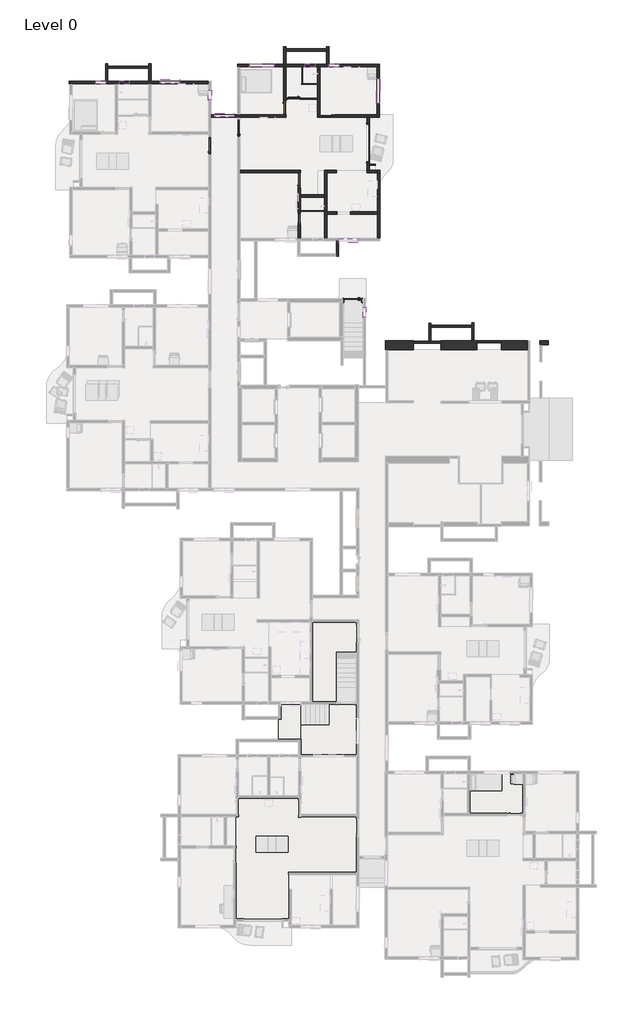
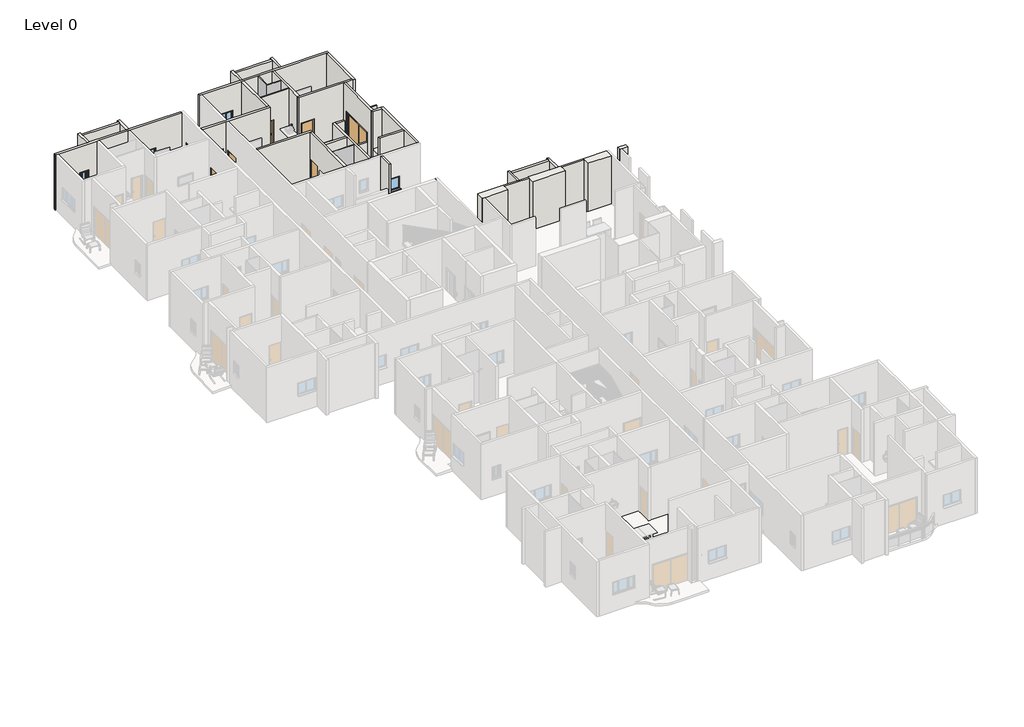
# One storey, part 7 of 14: 35 walls, 11 windows, 9 doors, 5 slabs, 3 plates.
"""IFC4 building model written with IfcOpenShell, lengths in millimetres."""

from ifc_helpers import new_model, si_unit, frame, origin, origin_with_axes, place, context, project, spatial, polyline, outline, extrude, faceted_brep, transform, mapped, element, save
from components import doors_concept_intdbl_8_5090a96f, doors_extsgl_flush_d1_30a970b5, doors_extsgl_flush_d1_11f69a25, doors_extsgl_flush_d2_fac1298c, doors_extsgl_flush_d2_5e0ff3e2, doors_extsgl_flush_d3_ba5ff989, doors_extsgl_flush_d3_b5fe9048, doors_intsgl_3_75_7d887cbf, system_panel_glazed_2e0a7f6c, system_panel_glazed_7dd01b14, system_panel_glazed_b430c16b, windows_concept_plain_dbl_4_d1e2e333, windows_sgl_plain_2_be143095, windows_tpl_variable_casement_2_47b04551, windows_tpl_variable_casement_2_4efd9f92, windows_tpl_variable_casement_5_ffad3fa3

model = new_model("IFC4")

# Units and contexts
model_context = context("Model", 3, world=origin())
ifc_project = project(units=[si_unit("LENGTHUNIT", "METRE", prefix="MILLI")], contexts=[model_context])

# Site, building, storey
site = spatial("IfcSite", under=ifc_project)
building = spatial("IfcBuilding", under=site)
storey = spatial("IfcBuildingStorey", under=building, Name="Level 0", Elevation=0.0)

# Doors
placement = place(None, origin())
doors_concept_intdbl_8_shape = doors_concept_intdbl_8_5090a96f(model_context)
element("IfcDoor", 1, ObjectType="Doors_Concept_IntDbl : 8'", at=placement, inside=storey, context=model_context, shape_type="MappedRepresentation", body=[
    mapped(doors_concept_intdbl_8_shape, transform((-21030.1788109, 60755.6698597, 0.0), x_axis=(0.0, -1.0, 0.0), y_axis=(1.0, 0.0, 0.0), z_axis=(0.0, 0.0, 1.0))),
])
doors_extsgl_flush_d1_shape = doors_extsgl_flush_d1_30a970b5(model_context)
element("IfcDoor", 2, ObjectType="Doors_ExtSgl_Flush : D1", at=placement, inside=storey, context=model_context, shape_type="MappedRepresentation", body=[
    mapped(doors_extsgl_flush_d1_shape, transform((-30896.1442282, 60598.8966557, 0.0), x_axis=(0.0, 1.0, 0.0), y_axis=(-1.0, 0.0, 0.0), z_axis=(0.0, 0.0, 1.0))),
])
doors_extsgl_flush_d1_2_shape = doors_extsgl_flush_d1_11f69a25(model_context)
element("IfcDoor", 3, ObjectType="Doors_ExtSgl_Flush : D1", at=placement, inside=storey, context=model_context, shape_type="MappedRepresentation", body=[
    mapped(doors_extsgl_flush_d1_2_shape, transform((-29094.6788109, 61678.6810361, 0.0), x_axis=(0.0, 1.0, 0.0), y_axis=(-1.0, 0.0, 0.0), z_axis=(0.0, 0.0, 1.0))),
])
doors_extsgl_flush_d2_shape = doors_extsgl_flush_d2_fac1298c(model_context)
element("IfcDoor", 4, ObjectType="Doors_ExtSgl_Flush : D2", at=placement, inside=storey, context=model_context, shape_type="MappedRepresentation", body=[
    mapped(doors_extsgl_flush_d2_shape, transform((-25322.6772109, 58440.0794361, 0.0), x_axis=(0.0, 1.0, 0.0), y_axis=(-1.0, 0.0, 0.0), z_axis=(0.0, 0.0, 1.0))),
])
doors_extsgl_flush_d2_2_shape = doors_extsgl_flush_d2_5e0ff3e2(model_context)
element("IfcDoor", 5, ObjectType="Doors_ExtSgl_Flush : D2", at=placement, inside=storey, context=model_context, shape_type="MappedRepresentation", body=[
    mapped(doors_extsgl_flush_d2_2_shape, transform((-23582.8144411, 62432.0698597, 0.0), x_axis=(-1.0, 0.0, 0.0), y_axis=(0.0, -1.0, 0.0), z_axis=(0.0, 0.0, 1.0))),
])
element("IfcDoor", 6, ObjectType="Doors_ExtSgl_Flush : D2", at=placement, inside=storey, context=model_context, shape_type="MappedRepresentation", body=[
    mapped(doors_extsgl_flush_d2_2_shape, transform((-26224.4144411, 62946.5795504, 0.0), x_axis=(0.0, -1.0, 0.0), y_axis=(1.0, 0.0, 0.0), z_axis=(0.0, 0.0, 1.0))),
])
doors_extsgl_flush_d3_shape = doors_extsgl_flush_d3_ba5ff989(model_context)
element("IfcDoor", 7, ObjectType="Doors_ExtSgl_Flush : D3", at=placement, inside=storey, context=model_context, shape_type="MappedRepresentation", body=[
    mapped(doors_extsgl_flush_d3_shape, transform((-25322.6772109, 56031.2698597, 0.0), x_axis=(0.0, 1.0, 0.0), y_axis=(-1.0, 0.0, 0.0), z_axis=(0.0, 0.0, 1.0))),
])
doors_extsgl_flush_d3_2_shape = doors_extsgl_flush_d3_b5fe9048(model_context)
element("IfcDoor", 8, ObjectType="Doors_ExtSgl_Flush : D3", at=placement, inside=storey, context=model_context, shape_type="MappedRepresentation", body=[
    mapped(doors_extsgl_flush_d3_2_shape, transform((-25640.2144411, 63519.8354932, 0.0), x_axis=(-1.0, 0.0, 0.0), y_axis=(0.0, -1.0, 0.0), z_axis=(0.0, 0.0, 1.0))),
])
doors_intsgl_3_75_shape = doors_intsgl_3_75_7d887cbf(model_context)
element("IfcDoor", 9, ObjectType="Doors_IntSgl : 3.75'", at=placement, inside=storey, context=model_context, shape_type="MappedRepresentation", body=[
    mapped(doors_intsgl_3_75_shape, transform((-21982.5772109, 50944.9706597, 0.0), x_axis=(-1.0, 0.0, 0.0), y_axis=(0.0, -1.0, 0.0), z_axis=(0.0, 0.0, 1.0))),
])

# Plates
system_panel_glazed_shape = system_panel_glazed_2e0a7f6c(model_context)
element("IfcPlate", 10, ObjectType="System Panel : Glazed", at=placement, inside=storey, context=model_context, shape_type="MappedRepresentation", body=[
    mapped(system_panel_glazed_shape, transform((-24497.1772109, 56563.0250546, 0.0), x_axis=(-1.0, 0.0, 0.0), y_axis=(0.0, -1.0, 0.0), z_axis=(0.0, 0.0, 1.0))),
])
system_panel_glazed_2_shape = system_panel_glazed_7dd01b14(model_context)
element("IfcPlate", 11, ObjectType="System Panel : Glazed", at=placement, inside=storey, context=model_context, shape_type="MappedRepresentation", body=[
    mapped(system_panel_glazed_2_shape, transform((-24687.7144411, 64484.3242932, 0.0), x_axis=(-1.0, 0.0, 0.0), y_axis=(0.0, -1.0, 0.0), z_axis=(0.0, 0.0, 1.0))),
])
system_panel_glazed_3_shape = system_panel_glazed_b430c16b(model_context)
element("IfcPlate", 12, ObjectType="System Panel : Glazed", at=placement, inside=storey, context=model_context, shape_type="MappedRepresentation", body=[
    mapped(system_panel_glazed_3_shape, transform((-25170.3144411, 65001.2978765, 0.0), x_axis=(0.0, 1.0, 0.0), y_axis=(-1.0, 0.0, 0.0), z_axis=(0.0, 0.0, 1.0))),
])

# Slabs
element("IfcSlab", 13, at=placement, inside=storey, context=model_context, shape_type="SweptSolid", body=[
    extrude(outline(polyline([(-25359.3553928, 19928.1411882), (-25359.3553928, 18745.0129431), (-21752.5553928, 18745.0129431), (-21752.5553928, 15341.4129431), (-25994.3553928, 15341.4129431), (-25994.3553928, 12426.7629431), (-29258.2553928, 12426.7629431), (-29258.2553928, 18745.0129431), (-29093.1553928, 18745.0129431), (-29093.1553928, 19928.1411882), (-25359.3553928, 19928.1411882)])), origin_with_axes(), (0.0, 0.0, 1.0), 149.9616),
])
element("IfcSlab", 14, ObjectType="OUTDOOR", at=placement, inside=storey, context=model_context, shape_type="SweptSolid", body=[
    extrude(outline(polyline([(-21744.3547508, 25782.7270746), (-21744.3547508, 22652.5601529), (-25206.9553928, 22652.5601529), (-25206.9553928, 24461.9270746), (-23446.1547508, 24461.9270746), (-23446.1547508, 25782.7270746), (-21744.3547508, 25782.7270746)])), frame((0.0, 0.0, 850.0384), z_axis=(0.0, 0.0, 1.0), x_axis=(1.0, 0.0, 0.0)), (0.0, 0.0, 1.0), 149.9616),
])
element("IfcSlab", 15, ObjectType="OUTDOOR", at=placement, inside=storey, context=model_context, shape_type="SweptSolid", body=[
    extrude(outline(polyline([(-26621.8300447, 23590.0629431), (-26621.8300447, 25782.7270746), (-25206.9553928, 25782.7270746), (-25206.9553928, 23590.0629431), (-26621.8300447, 23590.0629431)])), origin_with_axes(), (0.0, 0.0, 1.0), 149.9616),
])
element("IfcSlab", 16, ObjectType="STAIRCASE FLOORING", at=placement, inside=storey, context=model_context, shape_type="SweptSolid", body=[
    extrude(outline(polyline([(-21744.3547508, 30884.0294818), (-21744.3547508, 25935.1270746), (-24494.5800447, 25935.1270746), (-24494.5800447, 30884.0294818), (-21744.3547508, 30884.0294818)])), origin_with_axes(), (0.0, 0.0, 1.0), 149.9616),
])
element("IfcSlab", 17, ObjectType="STUDY ROOM", at=placement, inside=storey, context=model_context, shape_type="SweptSolid", body=[
    extrude(outline(polyline([(-11375.5465173, 21442.5122683), (-11375.5465173, 18997.7114683), (-14670.4537173, 18997.7114683), (-14670.4537173, 21442.5122683), (-11375.5465173, 21442.5122683)])), origin_with_axes(), (0.0, 0.0, 1.0), 149.9616),
])

# Walls
element("IfcWall", 18, ObjectType="W1", at=placement, inside=storey, context=model_context, shape_type="Brep", body=[
    faceted_brep([(-30972.3442282, 64612.2998557, 0.0), (-34554.8273605, 64612.2998557, 0.0), (-34707.2273605, 64612.2998557, 0.0), (-37254.3014709, 64612.2998557, 0.0), (-37406.7014709, 64612.2998557, 0.0), (-39671.9458282, 64612.2998557, 0.0), (-39671.9458282, 64612.2998557, 4000.0), (-37406.7014709, 64612.2998557, 4000.0), (-37254.3014709, 64612.2998557, 4000.0), (-34707.2273605, 64612.2998557, 4000.0), (-34554.8273605, 64612.2998557, 4000.0), (-30972.3442282, 64612.2998557, 4000.0), (-33996.0273605, 64612.2998557, 2110.0), (-33996.0273605, 64612.2998557, 1200.0), (-32776.8273605, 64612.2998557, 1200.0), (-32776.8273605, 64612.2998557, 2110.0), (-38003.4998709, 64612.2998557, 2110.0), (-38003.4998709, 64612.2998557, 1200.0), (-37393.8998709, 64612.2998557, 1200.0), (-37393.8998709, 64612.2998557, 2110.0), (-36530.2998709, 64612.2998557, 2738.9328), (-36530.2998709, 64612.2998557, 1828.9328), (-35920.6998709, 64612.2998557, 1828.9328), (-35920.6998709, 64612.2998557, 2738.9328), (-30972.3442282, 64459.8998557, 0.0), (-30972.3442282, 64459.8998557, 4000.0), (-34554.8273605, 64459.8998557, 4000.0), (-34707.2273605, 64459.8998557, 4000.0), (-36657.2998709, 64459.8998557, 4000.0), (-36809.6998709, 64459.8998557, 4000.0), (-39494.1458282, 64459.8998557, 4000.0), (-39646.5458282, 64459.8998557, 4000.0), (-39671.9458282, 64459.8998557, 4000.0), (-39671.9458282, 64459.8998557, 0.0), (-39646.5458282, 64459.8998557, 0.0), (-39494.1458282, 64459.8998557, 0.0), (-36809.6998709, 64459.8998557, 0.0), (-36657.2998709, 64459.8998557, 0.0), (-34707.2273605, 64459.8998557, 0.0), (-34554.8273605, 64459.8998557, 0.0), (-33996.0273605, 64459.8998557, 2110.0), (-32776.8273605, 64459.8998557, 2110.0), (-32776.8273605, 64459.8998557, 1200.0), (-33996.0273605, 64459.8998557, 1200.0), (-38003.4998709, 64459.8998557, 2110.0), (-37393.8998709, 64459.8998557, 2110.0), (-37393.8998709, 64459.8998557, 1200.0), (-38003.4998709, 64459.8998557, 1200.0), (-36530.2998709, 64459.8998557, 2738.9328), (-35920.6998709, 64459.8998557, 2738.9328), (-35920.6998709, 64459.8998557, 1828.9328), (-36530.2998709, 64459.8998557, 1828.9328)], [[[0, 1, 2, 3, 4, 5, 6, 7, 8, 9, 10, 11], [12, 13, 14, 15], [16, 17, 18, 19], [20, 21, 22, 23]], [[24, 25, 26, 27, 28, 29, 30, 31, 32, 33, 34, 35, 36, 37, 38, 39], [40, 41, 42, 43], [44, 45, 46, 47], [48, 49, 50, 51]], [[5, 4, 3, 2, 1, 0, 24, 39, 38, 37, 36, 35, 34, 33]], [[6, 5, 33, 32]], [[11, 10, 9, 8, 7, 6, 32, 31, 30, 29, 28, 27, 26, 25]], [[0, 11, 25, 24]], [[13, 12, 40, 43]], [[14, 13, 43, 42]], [[15, 14, 42, 41]], [[12, 15, 41, 40]], [[17, 16, 44, 47]], [[18, 17, 47, 46]], [[19, 18, 46, 45]], [[16, 19, 45, 44]], [[21, 20, 48, 51]], [[22, 21, 51, 50]], [[23, 22, 50, 49]], [[20, 23, 49, 48]]]),
])
element("IfcWall", 19, ObjectType="W1", at=placement, inside=storey, context=model_context, shape_type="Brep", body=[
    faceted_brep([(-37406.7014709, 65709.7127921, 0.0), (-37406.7014709, 64612.2998557, 0.0), (-37406.7014709, 64612.2998557, 4000.0), (-37406.7014709, 65709.7127921, 4000.0), (-37254.3014709, 65709.7127921, 0.0), (-37254.3014709, 65709.7127921, 4000.0), (-37254.3014709, 65557.3127921, 4000.0), (-37254.3014709, 65404.9127921, 4000.0), (-37254.3014709, 64612.2998557, 4000.0), (-37254.3014709, 64612.2998557, 0.0), (-37254.3014709, 65404.9127921, 0.0), (-37254.3014709, 65557.3127921, 0.0)], [[[0, 1, 2, 3]], [[4, 5, 6, 7, 8, 9, 10, 11]], [[1, 0, 4, 11, 10, 9]], [[3, 2, 8, 7, 6, 5]], [[0, 3, 5, 4]], [[2, 1, 9, 8]]]),
])
element("IfcWall", 20, ObjectType="W1", at=placement, inside=storey, context=model_context, shape_type="Brep", body=[
    faceted_brep([(-34707.2273605, 65706.4005109, 0.0), (-34707.2273605, 65557.3127921, 0.0), (-34707.2273605, 65404.9127921, 0.0), (-34707.2273605, 64612.2998557, 0.0), (-34707.2273605, 64612.2998557, 4000.0), (-34707.2273605, 65404.9127921, 4000.0), (-34707.2273605, 65557.3127921, 4000.0), (-34707.2273605, 65706.4005109, 4000.0), (-34554.8273605, 65706.4005109, 0.0), (-34554.8273605, 65706.4005109, 4000.0), (-34554.8273605, 64612.2998557, 4000.0), (-34554.8273605, 64612.2998557, 0.0)], [[[0, 1, 2, 3, 4, 5, 6, 7]], [[8, 9, 10, 11]], [[3, 2, 1, 0, 8, 11]], [[7, 6, 5, 4, 10, 9]], [[0, 7, 9, 8]], [[4, 3, 11, 10]]]),
])
element("IfcWall", 21, ObjectType="W1", at=placement, inside=storey, context=model_context, shape_type="Brep", body=[
    faceted_brep([(-30819.9442282, 62364.2982557, 0.0), (-29170.8788109, 62364.2982557, 0.0), (-29018.4788109, 62364.2982557, 0.0), (-26146.3442282, 62364.2982557, 0.0), (-26146.3442282, 62364.2982557, 4000.0), (-29018.4788109, 62364.2982557, 4000.0), (-29170.8788109, 62364.2982557, 4000.0), (-30819.9442282, 62364.2982557, 4000.0), (-30591.3442282, 62364.2982557, 2110.0), (-29372.1442282, 62364.2982557, 2110.0), (-29372.1442282, 62364.2982557, 1200.0), (-30591.3442282, 62364.2982557, 1200.0), (-26146.3442282, 62516.6982557, 4000.0), (-26146.3442282, 62516.6982557, 0.0), (-26148.2144411, 62516.6982557, 0.0), (-26148.2144411, 62516.6982557, 2110.0), (-26300.6144411, 62516.6982557, 2110.0), (-26313.4160411, 62516.6982557, 2110.0), (-26313.4160411, 62516.6982557, 0.0), (-29018.4788109, 62516.6982557, 0.0), (-29170.8788109, 62516.6982557, 0.0), (-30819.9442282, 62516.6982557, 0.0), (-30819.9442282, 62516.6982557, 4000.0), (-29170.8788109, 62516.6982557, 4000.0), (-29018.4788109, 62516.6982557, 4000.0), (-26300.6144411, 62516.6982557, 4000.0), (-26148.2144411, 62516.6982557, 4000.0), (-30591.3442282, 62516.6982557, 2110.0), (-30591.3442282, 62516.6982557, 1200.0), (-29372.1442282, 62516.6982557, 1200.0), (-29372.1442282, 62516.6982557, 2110.0), (-26313.4160411, 62489.3795504, 0.0), (-26148.2144411, 62489.3795504, 0.0), (-26313.4160411, 62489.3795504, 2110.0), (-26148.2144411, 62489.3795504, 2110.0)], [[[0, 1, 2, 3, 4, 5, 6, 7], [8, 9, 10, 11]], [[12, 13, 14, 15, 16, 17, 18, 19, 20, 21, 22, 23, 24, 25, 26], [27, 28, 29, 30]], [[3, 2, 1, 0, 21, 20, 19, 18, 31, 32, 14, 13]], [[4, 3, 13, 12]], [[7, 6, 5, 4, 12, 26, 25, 24, 23, 22]], [[0, 7, 22, 21]], [[33, 31, 18, 17]], [[32, 34, 15, 14]], [[31, 33, 34, 32]], [[34, 33, 17, 16, 15]], [[28, 27, 8, 11]], [[29, 28, 11, 10]], [[30, 29, 10, 9]], [[27, 30, 9, 8]]]),
])
element("IfcWall", 22, ObjectType="W1", at=placement, inside=storey, context=model_context, shape_type="Brep", body=[
    faceted_brep([(-20312.6288109, 65670.6714597, 0.0), (-23455.8144411, 65670.6714597, 0.0), (-23608.2144411, 65670.6714597, 0.0), (-26148.2144411, 65670.6714597, 0.0), (-26300.6144411, 65670.6714597, 0.0), (-29170.8788109, 65670.6714597, 0.0), (-29170.8788109, 65670.6714597, 4000.0), (-26300.6144411, 65670.6714597, 4000.0), (-26148.2144411, 65670.6714597, 4000.0), (-23608.2144411, 65670.6714597, 4000.0), (-23455.8144411, 65670.6714597, 4000.0), (-20312.6288109, 65670.6714597, 4000.0), (-28408.8788109, 65670.6714597, 2110.0), (-28408.8788109, 65670.6714597, 1200.0), (-26884.8788109, 65670.6714597, 1200.0), (-26884.8788109, 65670.6714597, 2110.0), (-23455.8144411, 65670.6714597, 2110.0), (-23455.8144411, 65670.6714597, 1200.0), (-22846.2144411, 65670.6714597, 1200.0), (-22846.2144411, 65670.6714597, 2110.0), (-24954.4144411, 65670.6714597, 2738.9328), (-24954.4144411, 65670.6714597, 1828.9328), (-24344.8144411, 65670.6714597, 1828.9328), (-24344.8144411, 65670.6714597, 2738.9328), (-20312.6288109, 65518.2714597, 0.0), (-20312.6288109, 65518.2714597, 4000.0), (-20465.0288109, 65518.2714597, 4000.0), (-24040.0144411, 65518.2714597, 4000.0), (-24192.4144411, 65518.2714597, 4000.0), (-26148.2144411, 65518.2714597, 4000.0), (-26300.6144411, 65518.2714597, 4000.0), (-29018.4788109, 65518.2714597, 4000.0), (-29170.8788109, 65518.2714597, 4000.0), (-29170.8788109, 65518.2714597, 0.0), (-29018.4788109, 65518.2714597, 0.0), (-26300.6144411, 65518.2714597, 0.0), (-26148.2144411, 65518.2714597, 0.0), (-24192.4144411, 65518.2714597, 0.0), (-24040.0144411, 65518.2714597, 0.0), (-20465.0288109, 65518.2714597, 0.0), (-28408.8788109, 65518.2714597, 2110.0), (-26884.8788109, 65518.2714597, 2110.0), (-26884.8788109, 65518.2714597, 1200.0), (-28408.8788109, 65518.2714597, 1200.0), (-23455.8144411, 65518.2714597, 2110.0), (-22846.2144411, 65518.2714597, 2110.0), (-22846.2144411, 65518.2714597, 1200.0), (-23455.8144411, 65518.2714597, 1200.0), (-24954.4144411, 65518.2714597, 2738.9328), (-24344.8144411, 65518.2714597, 2738.9328), (-24344.8144411, 65518.2714597, 1828.9328), (-24954.4144411, 65518.2714597, 1828.9328)], [[[0, 1, 2, 3, 4, 5, 6, 7, 8, 9, 10, 11], [12, 13, 14, 15], [16, 17, 18, 19], [20, 21, 22, 23]], [[24, 25, 26, 27, 28, 29, 30, 31, 32, 33, 34, 35, 36, 37, 38, 39], [40, 41, 42, 43], [44, 45, 46, 47], [48, 49, 50, 51]], [[5, 4, 3, 2, 1, 0, 24, 39, 38, 37, 36, 35, 34, 33]], [[11, 10, 9, 8, 7, 6, 32, 31, 30, 29, 28, 27, 26, 25]], [[0, 11, 25, 24]], [[6, 5, 33, 32]], [[13, 12, 40, 43]], [[14, 13, 43, 42]], [[15, 14, 42, 41]], [[12, 15, 41, 40]], [[17, 16, 44, 47]], [[18, 17, 47, 46]], [[19, 18, 46, 45]], [[16, 19, 45, 44]], [[21, 20, 48, 51]], [[22, 21, 51, 50]], [[23, 22, 50, 49]], [[20, 23, 49, 48]]]),
])
element("IfcWall", 23, ObjectType="W1", at=placement, inside=storey, context=model_context, shape_type="Brep", body=[
    faceted_brep([(-20465.0288109, 65518.2714597, 0.0), (-20465.0288109, 62508.2698597, 0.0), (-20465.0288109, 62355.8698597, 0.0), (-20465.0288109, 62355.8698597, 4000.0), (-20465.0288109, 62508.2698597, 4000.0), (-20465.0288109, 65518.2714597, 4000.0), (-20465.0288109, 64775.2706597, 2110.0), (-20465.0288109, 63251.2706597, 2110.0), (-20465.0288109, 63251.2706597, 1200.0), (-20465.0288109, 64775.2706597, 1200.0), (-20312.6288109, 65518.2714597, 0.0), (-20312.6288109, 65518.2714597, 4000.0), (-20312.6288109, 62355.8698597, 4000.0), (-20312.6288109, 62355.8698597, 0.0), (-20312.6288109, 64775.2706597, 2110.0), (-20312.6288109, 64775.2706597, 1200.0), (-20312.6288109, 63251.2706597, 1200.0), (-20312.6288109, 63251.2706597, 2110.0)], [[[0, 1, 2, 3, 4, 5], [6, 7, 8, 9]], [[10, 11, 12, 13], [14, 15, 16, 17]], [[2, 1, 0, 10, 13]], [[5, 4, 3, 12, 11]], [[0, 5, 11, 10]], [[3, 2, 13, 12]], [[15, 14, 6, 9]], [[16, 15, 9, 8]], [[17, 16, 8, 7]], [[14, 17, 7, 6]]]),
])
element("IfcWall", 24, ObjectType="W1", at=placement, inside=storey, context=model_context, shape_type="Brep", body=[
    faceted_brep([(-24040.0144411, 62508.2698597, 2110.0), (-24040.0144411, 62508.2698597, 0.0), (-24192.4144411, 62508.2698597, 0.0), (-24192.4144411, 62508.2698597, 4000.0), (-24040.0144411, 62508.2698597, 4000.0), (-20465.0288109, 62508.2698597, 4000.0), (-20465.0288109, 62508.2698597, 0.0), (-23125.6144411, 62508.2698597, 0.0), (-23125.6144411, 62508.2698597, 2110.0), (-24192.4144411, 62355.8698597, 0.0), (-24040.0144411, 62355.8698597, 0.0), (-24040.0144411, 62355.8698597, 2110.0), (-23125.6144411, 62355.8698597, 2110.0), (-23125.6144411, 62355.8698597, 0.0), (-21106.3788109, 62355.8698597, 0.0), (-20953.9788109, 62355.8698597, 0.0), (-20465.0288109, 62355.8698597, 0.0), (-20465.0288109, 62355.8698597, 4000.0), (-20953.9788109, 62355.8698597, 4000.0), (-21106.3788109, 62355.8698597, 4000.0), (-24192.4144411, 62355.8698597, 4000.0)], [[[0, 1, 2, 3, 4, 5, 6, 7, 8]], [[9, 10, 11, 12, 13, 14, 15, 16, 17, 18, 19, 20]], [[7, 6, 16, 15, 14, 13]], [[2, 1, 10, 9]], [[5, 4, 3, 20, 19, 18, 17]], [[6, 5, 17, 16]], [[3, 2, 9, 20]], [[13, 12, 8, 7]], [[11, 10, 1, 0]], [[12, 11, 0, 8]]]),
])
element("IfcWall", 25, ObjectType="W1", at=placement, inside=storey, context=model_context, shape_type="Brep", body=[
    faceted_brep([(-26300.6144411, 66770.3242932, 4000.0), (-26300.6144411, 66770.3242932, 0.0), (-26300.6144411, 65670.6714597, 0.0), (-26300.6144411, 65670.6714597, 4000.0), (-26148.2144411, 66770.3242932, 0.0), (-26148.2144411, 66770.3242932, 4000.0), (-26148.2144411, 66617.9242932, 4000.0), (-26148.2144411, 66465.5242932, 4000.0), (-26148.2144411, 65670.6714597, 4000.0), (-26148.2144411, 65670.6714597, 0.0), (-26148.2144411, 66465.5242932, 0.0), (-26148.2144411, 66617.9242932, 0.0)], [[[0, 1, 2, 3]], [[4, 5, 6, 7, 8, 9, 10, 11]], [[1, 4, 11, 10, 9, 2]], [[5, 0, 3, 8, 7, 6]], [[1, 0, 5, 4]], [[3, 2, 9, 8]]]),
    faceted_brep([(-26300.6144411, 62516.6982557, 2110.0), (-26300.6144411, 62516.6982557, 4000.0), (-26300.6144411, 65518.2714597, 4000.0), (-26300.6144411, 65518.2714597, 0.0), (-26300.6144411, 63403.7795504, 0.0), (-26300.6144411, 63403.7795504, 2110.0), (-26148.2144411, 62516.6982557, 4000.0), (-26148.2144411, 62516.6982557, 2110.0), (-26148.2144411, 63403.7795504, 2110.0), (-26148.2144411, 63403.7795504, 0.0), (-26148.2144411, 63495.1466932, 0.0), (-26148.2144411, 63544.5242932, 0.0), (-26148.2144411, 65518.2714597, 0.0), (-26148.2144411, 65518.2714597, 4000.0), (-26148.2144411, 63544.5242932, 4000.0), (-26148.2144411, 63495.1466932, 4000.0)], [[[0, 1, 2, 3, 4, 5]], [[6, 7, 8, 9, 10, 11, 12, 13, 14, 15]], [[9, 4, 3, 12, 11, 10]], [[1, 6, 15, 14, 13, 2]], [[3, 2, 13, 12]], [[6, 1, 0, 7]], [[8, 5, 4, 9]], [[5, 8, 7, 0]]]),
])
element("IfcWall", 26, ObjectType="W1", at=placement, inside=storey, context=model_context, shape_type="Brep", body=[
    faceted_brep([(-24192.4144411, 65518.2714597, 0.0), (-24192.4144411, 63544.5242932, 0.0), (-24192.4144411, 63495.1466932, 0.0), (-24192.4144411, 62508.2698597, 0.0), (-24192.4144411, 62508.2698597, 4000.0), (-24192.4144411, 63495.1466932, 4000.0), (-24192.4144411, 63544.5242932, 4000.0), (-24192.4144411, 65518.2714597, 4000.0), (-24040.0144411, 65518.2714597, 0.0), (-24040.0144411, 65518.2714597, 4000.0), (-24040.0144411, 62508.2698597, 4000.0), (-24040.0144411, 62508.2698597, 2110.0), (-24040.0144411, 62508.2698597, 0.0)], [[[0, 1, 2, 3, 4, 5, 6, 7]], [[8, 9, 10, 11, 12]], [[3, 2, 1, 0, 8, 12]], [[7, 6, 5, 4, 10, 9]], [[4, 3, 12, 11, 10]], [[0, 7, 9, 8]]]),
])
element("IfcWall", 27, ObjectType="W1", at=placement, inside=storey, context=model_context, shape_type="Brep", body=[
    faceted_brep([(-29018.4788109, 58910.0810361, 0.0), (-25398.8772109, 58910.0810361, 0.0), (-25246.4772109, 58910.0810361, 0.0), (-25246.4772109, 58910.0810361, 4000.0), (-25398.8772109, 58910.0810361, 4000.0), (-29018.4788109, 58910.0810361, 4000.0), (-29018.4788109, 59062.4810361, 0.0), (-29018.4788109, 59062.4810361, 4000.0), (-25246.4772109, 59062.4810361, 4000.0), (-25246.4772109, 59062.4810361, 0.0)], [[[0, 1, 2, 3, 4, 5]], [[6, 7, 8, 9]], [[2, 1, 0, 6, 9]], [[5, 4, 3, 8, 7]], [[0, 5, 7, 6]], [[3, 2, 9, 8]]]),
])
element("IfcWall", 28, ObjectType="W1", at=placement, inside=storey, context=model_context, shape_type="Brep", body=[
    faceted_brep([(-25246.4772109, 56412.2698597, 2110.0), (-25246.4772109, 56412.2698597, 0.0), (-25246.4772109, 57373.2794361, 0.0), (-25246.4772109, 57525.6794361, 0.0), (-25246.4772109, 57982.8794361, 0.0), (-25246.4772109, 57982.8794361, 2110.0), (-25246.4772109, 58897.2794361, 2110.0), (-25246.4772109, 58897.2794361, 0.0), (-25246.4772109, 58910.0810361, 0.0), (-25246.4772109, 58910.0810361, 4000.0), (-25246.4772109, 57525.6794361, 4000.0), (-25246.4772109, 57373.2794361, 4000.0), (-25246.4772109, 54812.0698597, 4000.0), (-25246.4772109, 54812.0698597, 0.0), (-25246.4772109, 55650.2698597, 0.0), (-25246.4772109, 55650.2698597, 2110.0), (-25398.8772109, 57982.8794361, 0.0), (-25398.8772109, 56412.2698597, 0.0), (-25398.8772109, 56412.2698597, 2110.0), (-25398.8772109, 55650.2698597, 2110.0), (-25398.8772109, 55650.2698597, 0.0), (-25398.8772109, 54812.0698597, 0.0), (-25398.8772109, 54812.0698597, 4000.0), (-25398.8772109, 58910.0810361, 4000.0), (-25398.8772109, 58910.0810361, 0.0), (-25398.8772109, 58897.2794361, 0.0), (-25398.8772109, 58897.2794361, 2110.0), (-25398.8772109, 57982.8794361, 2110.0)], [[[0, 1, 2, 3, 4, 5, 6, 7, 8, 9, 10, 11, 12, 13, 14, 15]], [[16, 17, 18, 19, 20, 21, 22, 23, 24, 25, 26, 27]], [[24, 8, 7, 25]], [[14, 13, 21, 20]], [[4, 3, 2, 1, 17, 16]], [[12, 11, 10, 9, 23, 22]], [[9, 8, 24, 23]], [[13, 12, 22, 21]], [[27, 5, 4, 16]], [[6, 26, 25, 7]], [[5, 27, 26, 6]], [[20, 19, 15, 14]], [[18, 17, 1, 0]], [[19, 18, 0, 15]]]),
])
element("IfcWall", 29, ObjectType="W1", at=placement, inside=storey, context=model_context, shape_type="Brep", body=[
    faceted_brep([(-23595.4772109, 54812.0698597, 0.0), (-23595.4772109, 56309.0250546, 0.0), (-23595.4772109, 56461.4250546, 0.0), (-23595.4772109, 58910.0810361, 0.0), (-23595.4772109, 59062.4810361, 0.0), (-23595.4772109, 59062.4810361, 4000.0), (-23595.4772109, 58910.0810361, 4000.0), (-23595.4772109, 56461.4250546, 4000.0), (-23595.4772109, 56309.0250546, 4000.0), (-23595.4772109, 54812.0698597, 4000.0), (-23747.8772109, 54812.0698597, 0.0), (-23747.8772109, 54812.0698597, 4000.0), (-23747.8772109, 57373.2794361, 4000.0), (-23747.8772109, 57525.6794361, 4000.0), (-23747.8772109, 59062.4810361, 4000.0), (-23747.8772109, 59062.4810361, 0.0), (-23747.8772109, 57525.6794361, 0.0), (-23747.8772109, 57373.2794361, 0.0)], [[[0, 1, 2, 3, 4, 5, 6, 7, 8, 9]], [[10, 11, 12, 13, 14, 15, 16, 17]], [[4, 3, 2, 1, 0, 10, 17, 16, 15]], [[9, 8, 7, 6, 5, 14, 13, 12, 11]], [[0, 9, 11, 10]], [[5, 4, 15, 14]]]),
])
element("IfcWall", 30, ObjectType="W1", at=placement, inside=storey, context=model_context, shape_type="SweptSolid", body=[
    extrude(outline(polyline([(-23747.8772109, 57373.2794361), (-25246.4772109, 57373.2794361), (-25246.4772109, 57525.6794361), (-23747.8772109, 57525.6794361), (-23747.8772109, 57373.2794361)])), origin_with_axes(), (0.0, 0.0, 1.0), 4000.0),
])
element("IfcWall", 31, ObjectType="W1", at=placement, inside=storey, context=model_context, shape_type="Brep", body=[
    faceted_brep([(-20293.4772109, 54812.0698597, 0.0), (-20293.4772109, 59053.8698597, 0.0), (-20293.4772109, 59053.8698597, 4000.0), (-20293.4772109, 54812.0698597, 4000.0), (-20445.8772109, 54812.0698597, 0.0), (-20445.8772109, 54812.0698597, 4000.0), (-20445.8772109, 56309.0250546, 4000.0), (-20445.8772109, 56461.4250546, 4000.0), (-20445.8772109, 58901.4698597, 4000.0), (-20445.8772109, 59053.8698597, 4000.0), (-20445.8772109, 59053.8698597, 0.0), (-20445.8772109, 58901.4698597, 0.0), (-20445.8772109, 56461.4250546, 0.0), (-20445.8772109, 56309.0250546, 0.0)], [[[0, 1, 2, 3]], [[4, 5, 6, 7, 8, 9, 10, 11, 12, 13]], [[1, 0, 4, 13, 12, 11, 10]], [[3, 2, 9, 8, 7, 6, 5]], [[0, 3, 5, 4]], [[2, 1, 10, 9]]]),
])
element("IfcWall", 32, ObjectType="W1", at=placement, inside=storey, context=model_context, shape_type="SweptSolid", body=[
    extrude(outline(polyline([(-23011.2772109, 58910.0810361), (-23595.4772109, 58910.0810361), (-23595.4772109, 59062.4810361), (-23011.2772109, 59062.4810361), (-23011.2772109, 58910.0810361)])), origin_with_axes(), (0.0, 0.0, 1.0), 4000.0),
])
element("IfcWall", 33, ObjectType="W1", at=placement, inside=storey, context=model_context, shape_type="Brep", body=[
    faceted_brep([(-20445.8772109, 59053.8698597, 0.0), (-20953.9788109, 59053.8698597, 0.0), (-21106.3788109, 59053.8698597, 0.0), (-21106.3788109, 59053.8698597, 4000.0), (-20953.9788109, 59053.8698597, 4000.0), (-20445.8772109, 59053.8698597, 4000.0), (-20445.8772109, 58901.4698597, 0.0), (-20445.8772109, 58901.4698597, 4000.0), (-21106.3788109, 58901.4698597, 4000.0), (-21106.3788109, 58901.4698597, 0.0)], [[[0, 1, 2, 3, 4, 5]], [[6, 7, 8, 9]], [[2, 1, 0, 6, 9]], [[5, 4, 3, 8, 7]], [[0, 5, 7, 6]], [[3, 2, 9, 8]]]),
])
element("IfcWall", 34, ObjectType="W1", at=placement, inside=storey, context=model_context, shape_type="Brep", body=[
    faceted_brep([(-20953.9788109, 62355.8698597, 4000.0), (-20953.9788109, 59434.8698597, 4000.0), (-20953.9788109, 59385.4922597, 4000.0), (-20953.9788109, 59053.8698597, 4000.0), (-20953.9788109, 59053.8698597, 0.0), (-20953.9788109, 59385.4922597, 0.0), (-20953.9788109, 59434.8698597, 0.0), (-20953.9788109, 59536.4698597, 0.0), (-20953.9788109, 59536.4698597, 2110.0), (-20953.9788109, 61974.8698597, 2110.0), (-20953.9788109, 61974.8698597, 0.0), (-20953.9788109, 62355.8698597, 0.0), (-21106.3788109, 59053.8698597, 4000.0), (-21106.3788109, 62355.8698597, 4000.0), (-21106.3788109, 62355.8698597, 0.0), (-21106.3788109, 61974.8698597, 0.0), (-21106.3788109, 61974.8698597, 2110.0), (-21106.3788109, 59536.4698597, 2110.0), (-21106.3788109, 59536.4698597, 0.0), (-21106.3788109, 59053.8698597, 0.0)], [[[0, 1, 2, 3, 4, 5, 6, 7, 8, 9, 10, 11]], [[12, 13, 14, 15, 16, 17, 18, 19]], [[4, 19, 18, 7, 6, 5]], [[14, 11, 10, 15]], [[3, 2, 1, 0, 13, 12]], [[4, 3, 12, 19]], [[0, 11, 14, 13]], [[17, 8, 7, 18]], [[8, 17, 16, 9]], [[9, 16, 15, 10]]]),
])
element("IfcWall", 35, ObjectType="W1", at=placement, inside=storey, context=model_context, shape_type="Brep", body=[
    faceted_brep([(-23011.2772109, 54659.6698597, 0.0), (-23011.2772109, 53859.4682597, 0.0), (-23011.2772109, 53707.0682597, 0.0), (-23011.2772109, 53707.0682597, 2171.2), (-23011.2772109, 53707.0682597, 4000.0), (-23011.2772109, 54659.6698597, 4000.0), (-22858.8772109, 54659.6698597, 0.0), (-22858.8772109, 54659.6698597, 4000.0), (-22858.8772109, 53707.0682597, 4000.0), (-22858.8772109, 53707.0682597, 0.0)], [[[0, 1, 2, 3, 4, 5]], [[6, 7, 8, 9]], [[2, 1, 0, 6, 9]], [[5, 4, 8, 7]], [[0, 5, 7, 6]], [[4, 3, 2, 9, 8]]]),
])
element("IfcWall", 36, ObjectType="W1", at=placement, inside=storey, context=model_context, shape_type="Brep", body=[
    faceted_brep([(-23455.8144411, 65670.6714597, 0.0), (-23455.8144411, 66762.8714597, 0.0), (-23455.8144411, 66762.8714597, 4000.0), (-23455.8144411, 65670.6714597, 4000.0), (-23455.8144411, 65670.6714597, 2110.0), (-23455.8144411, 65670.6714597, 1200.0), (-23608.2144411, 65670.6714597, 0.0), (-23608.2144411, 65670.6714597, 4000.0), (-23608.2144411, 66465.5242932, 4000.0), (-23608.2144411, 66617.9242932, 4000.0), (-23608.2144411, 66762.8714597, 4000.0), (-23608.2144411, 66762.8714597, 0.0), (-23608.2144411, 66617.9242932, 0.0), (-23608.2144411, 66465.5242932, 0.0)], [[[0, 1, 2, 3, 4, 5]], [[6, 7, 8, 9, 10, 11, 12, 13]], [[1, 0, 6, 13, 12, 11]], [[2, 1, 11, 10]], [[3, 2, 10, 9, 8, 7]], [[0, 5, 4, 3, 7, 6]]]),
])
element("IfcWall", 37, ObjectType="W1", at=placement, inside=storey, context=model_context, shape_type="SweptSolid", body=[
    extrude(outline(polyline([(-22122.2772109, 56461.4250546), (-20445.8772109, 56461.4250546), (-20445.8772109, 56309.0250546), (-22122.2772109, 56309.0250546), (-22122.2772109, 56461.4250546)])), origin_with_axes(), (0.0, 0.0, 1.0), 4000.0),
])
element("IfcWall", 38, ObjectType="W1", at=placement, inside=storey, context=model_context, shape_type="SweptSolid", body=[
    extrude(outline(polyline([(-23595.4772109, 56461.4250546), (-22960.4772109, 56461.4250546), (-22960.4772109, 56309.0250546), (-23595.4772109, 56309.0250546), (-23595.4772109, 56461.4250546)])), origin_with_axes(), (0.0, 0.0, 1.0), 4000.0),
])
element("IfcWall", 39, ObjectType="W1", at=placement, inside=storey, context=model_context, shape_type="SweptSolid", body=[
    extrude(outline(polyline([(-17107.4265132, 49417.5165308), (-14539.5134669, 49417.5165308), (-14539.5134669, 49265.1165308), (-17107.4265132, 49265.1165308), (-17107.4265132, 49417.5165308)])), origin_with_axes(), (0.0, 0.0, 1.0), 4000.0),
])
element("IfcWall", 40, ObjectType="W1", at=placement, inside=storey, context=model_context, shape_type="SweptSolid", body=[
    extrude(outline(polyline([(-34707.2273605, 65404.9127921), (-37254.3014709, 65404.9127921), (-37254.3014709, 65557.3127921), (-34707.2273605, 65557.3127921), (-34707.2273605, 65404.9127921)])), origin_with_axes(), (0.0, 0.0, 1.0), 4000.0),
])
element("IfcWall", 41, ObjectType="W1", at=placement, inside=storey, context=model_context, shape_type="SweptSolid", body=[
    extrude(outline(polyline([(-23608.2144411, 66465.5242932), (-26148.2144411, 66465.5242932), (-26148.2144411, 66617.9242932), (-23608.2144411, 66617.9242932), (-23608.2144411, 66465.5242932)])), origin_with_axes(), (0.0, 0.0, 1.0), 4000.0),
])
element("IfcWall", 42, ObjectType="W2", at=placement, inside=storey, context=model_context, shape_type="SweptSolid", body=[
    extrude(outline(polyline([(0.0, -26148.2144411), (0.0, -26021.2144411), (2110.0, -26021.2144411), (2110.0, -25259.2144411), (0.0, -25259.2144411), (0.0, -24192.4144411), (4000.0, -24192.4144411), (4000.0, -26148.2144411), (0.0, -26148.2144411)])), frame((0.0, 63495.1466932, 0.0), z_axis=(0.0, 1.0, 0.0), x_axis=(0.0, 0.0, 1.0)), (0.0, 0.0, 1.0), 49.3776),
])
element("IfcWall", 43, ObjectType="W2", at=placement, inside=storey, context=model_context, shape_type="SweptSolid", body=[
    extrude(outline(polyline([(-20560.1772109, 59385.4922597), (-20953.9788109, 59385.4922597), (-20953.9788109, 59434.8698597), (-20560.1772109, 59434.8698597), (-20560.1772109, 59385.4922597)])), origin_with_axes(), (0.0, 0.0, 1.0), 4000.0),
])
element("IfcWall", 44, ObjectType="W3", at=placement, inside=storey, context=model_context, shape_type="Brep", body=[
    faceted_brep([(-10328.7145289, 48181.1171358, 0.0), (-10201.6129289, 48181.1171358, 0.0), (-9769.9145289, 48181.1171358, 0.0), (-9769.9145289, 48181.1171358, 4000.0), (-10201.6129289, 48181.1171358, 4000.0), (-10328.7145289, 48181.1171358, 4000.0), (-10328.7145289, 48441.4163358, 0.0), (-10328.7145289, 48441.4163358, 4000.0), (-9769.9145289, 48441.4163358, 4000.0), (-9769.9145289, 48441.4163358, 0.0)], [[[0, 1, 2, 3, 4, 5]], [[6, 7, 8, 9]], [[2, 1, 0, 6, 9]], [[3, 2, 9, 8]], [[5, 4, 3, 8, 7]], [[0, 5, 7, 6]]]),
])
element("IfcWall", 45, ObjectType="W6", at=placement, inside=storey, context=model_context, shape_type="SweptSolid", body=[
    extrude(outline(polyline([(-21319.9304686, 50918.084279), (-21357.9288686, 50918.084279), (-21357.9288686, 51045.185879), (-21319.9304686, 51045.185879), (-21319.9304686, 50918.084279)])), origin_with_axes(), (0.0, 0.0, 1.0), 4000.0),
])
element("IfcWall", 46, ObjectType="W6", at=placement, inside=storey, context=model_context, shape_type="Brep", body=[
    faceted_brep([(-17234.5281132, 49537.3010865, 0.0), (-17234.5281132, 48413.708507, 0.0), (-17234.5281132, 48413.708507, 4000.0), (-17234.5281132, 49537.3010865, 4000.0), (-17107.4265132, 49537.3010865, 0.0), (-17107.4265132, 49537.3010865, 4000.0), (-17107.4265132, 49417.5165308, 4000.0), (-17107.4265132, 49265.1165308, 4000.0), (-17107.4265132, 48413.708507, 4000.0), (-17107.4265132, 48413.708507, 0.0), (-17107.4265132, 49265.1165308, 0.0), (-17107.4265132, 49417.5165308, 0.0)], [[[0, 1, 2, 3]], [[4, 5, 6, 7, 8, 9, 10, 11]], [[1, 0, 4, 11, 10, 9]], [[3, 2, 8, 7, 6, 5]], [[0, 3, 5, 4]], [[2, 1, 9, 8]]]),
])
element("IfcWall", 47, ObjectType="W6", at=placement, inside=storey, context=model_context, shape_type="Brep", body=[
    faceted_brep([(-14539.5134669, 49544.5165308, 0.0), (-14539.5134669, 49417.5165308, 0.0), (-14539.5134669, 49265.1165308, 0.0), (-14539.5134669, 48432.758507, 0.0), (-14539.5134669, 48432.758507, 4000.0), (-14539.5134669, 49265.1165308, 4000.0), (-14539.5134669, 49417.5165308, 4000.0), (-14539.5134669, 49544.5165308, 4000.0), (-14412.4118669, 49544.5165308, 0.0), (-14412.4118669, 49544.5165308, 4000.0), (-14412.4118669, 48432.758507, 4000.0), (-14412.4118669, 48432.758507, 0.0)], [[[0, 1, 2, 3, 4, 5, 6, 7]], [[8, 9, 10, 11]], [[3, 2, 1, 0, 8, 11]], [[7, 6, 5, 4, 10, 9]], [[0, 7, 9, 8]], [[4, 3, 11, 10]]]),
])
element("IfcWall", 48, ObjectType="W6", at=placement, inside=storey, context=model_context, shape_type="SweptSolid", body=[
    extrude(outline(polyline([(-12710.6118669, 48299.8149308), (-14234.6118669, 48299.8149308), (-14234.6118669, 48426.9165308), (-12710.6118669, 48426.9165308), (-12710.6118669, 48299.8149308)])), origin_with_axes(), (0.0, 0.0, 1.0), 4000.0),
])
element("IfcWall", 49, ObjectType="W6", at=placement, inside=storey, context=model_context, shape_type="Brep", body=[
    faceted_brep([(-18183.500235, 48286.606907, 0.0), (-16481.700235, 48286.606907, 0.0), (-16481.700235, 48286.606907, 4000.0), (-18183.500235, 48286.606907, 4000.0), (-18183.500235, 48413.708507, 0.0), (-18183.500235, 48413.708507, 4000.0), (-17234.5281132, 48413.708507, 4000.0), (-17107.4265132, 48413.708507, 4000.0), (-16481.700235, 48413.708507, 4000.0), (-16481.700235, 48413.708507, 0.0), (-17107.4265132, 48413.708507, 0.0), (-17234.5281132, 48413.708507, 0.0)], [[[0, 1, 2, 3]], [[4, 5, 6, 7, 8, 9, 10, 11]], [[1, 0, 4, 11, 10, 9]], [[2, 1, 9, 8]], [[3, 2, 8, 7, 6, 5]], [[0, 3, 5, 4]]]),
])
element("IfcWall", 50, ObjectType="W7", at=placement, inside=storey, context=model_context, shape_type="Brep", body=[
    faceted_brep([(-19935.5870717, 47870.1159129, 0.0), (-19922.1391841, 47870.1159129, 0.0), (-19795.0375841, 47870.1159129, 0.0), (-18183.500235, 47870.1159129, 0.0), (-18183.500235, 47870.1159129, 4000.0), (-19795.0375841, 47870.1159129, 4000.0), (-19922.1391841, 47870.1159129, 4000.0), (-19935.5870717, 47870.1159129, 4000.0), (-19935.5870717, 48428.8143129, 0.0), (-19935.5870717, 48428.8143129, 4000.0), (-18183.500235, 48428.8143129, 4000.0), (-18183.500235, 48428.8143129, 0.0), (-18183.500235, 48413.708507, 0.0), (-18183.500235, 48286.606907, 0.0), (-18183.500235, 48413.708507, 4000.0), (-18183.500235, 48286.606907, 4000.0)], [[[0, 1, 2, 3, 4, 5, 6, 7]], [[8, 9, 10, 11]], [[3, 2, 1, 0, 8, 11, 12, 13]], [[4, 3, 13, 12, 11, 10, 14, 15]], [[7, 6, 5, 4, 15, 14, 10, 9]], [[0, 7, 9, 8]]]),
])
element("IfcWall", 51, ObjectType="W7", at=placement, inside=storey, context=model_context, shape_type="Brep", body=[
    faceted_brep([(-16481.700235, 47874.060107, 0.0), (-14234.6118669, 47874.060107, 0.0), (-14234.6118669, 47874.060107, 4000.0), (-16481.700235, 47874.060107, 4000.0), (-16481.700235, 48432.758507, 0.0), (-16481.700235, 48432.758507, 4000.0), (-14539.5134669, 48432.758507, 4000.0), (-14412.4118669, 48432.758507, 4000.0), (-14234.6118669, 48432.758507, 4000.0), (-14234.6118669, 48432.758507, 0.0), (-14412.4118669, 48432.758507, 0.0), (-14539.5134669, 48432.758507, 0.0), (-16481.700235, 48286.606907, 0.0), (-16481.700235, 48413.708507, 0.0), (-14234.6118669, 48426.9165308, 0.0), (-14234.6118669, 48299.8149308, 0.0), (-14234.6118669, 48426.9165308, 4000.0), (-14234.6118669, 48299.8149308, 4000.0), (-16481.700235, 48413.708507, 4000.0), (-16481.700235, 48286.606907, 4000.0)], [[[0, 1, 2, 3]], [[4, 5, 6, 7, 8, 9, 10, 11]], [[1, 0, 12, 13, 4, 11, 10, 9, 14, 15]], [[2, 1, 15, 14, 9, 8, 16, 17]], [[3, 2, 17, 16, 8, 7, 6, 5, 18, 19]], [[0, 3, 19, 18, 5, 4, 13, 12]]]),
])
element("IfcWall", 52, ObjectType="W7", at=placement, inside=storey, context=model_context, shape_type="Brep", body=[
    faceted_brep([(-12710.6118669, 47868.2181308, 0.0), (-11074.6610598, 47868.2181308, 0.0), (-11074.6610598, 47868.2181308, 4000.0), (-12710.6118669, 47868.2181308, 4000.0), (-12710.6118669, 48426.9165308, 0.0), (-12710.6118669, 48426.9165308, 4000.0), (-11074.6610598, 48426.9165308, 4000.0), (-11074.6610598, 48426.9165308, 0.0), (-12710.6118669, 48299.8149308, 0.0), (-12710.6118669, 48299.8149308, 4000.0)], [[[0, 1, 2, 3]], [[4, 5, 6, 7]], [[1, 0, 8, 4, 7]], [[3, 2, 6, 5, 9]], [[0, 3, 9, 5, 4, 8]], [[2, 1, 7, 6]]]),
])

# Windows
windows_concept_plain_dbl_4_shape = windows_concept_plain_dbl_4_d1e2e333(model_context)
element("IfcWindow", 53, ObjectType="Windows_Concept_Plain_Dbl : 4'", at=placement, inside=storey, context=model_context, shape_type="MappedRepresentation", body=[
    mapped(windows_concept_plain_dbl_4_shape, transform((-22559.6772109, 54744.3264275, 0.0), x_axis=(-1.0, 0.0, 0.0), y_axis=(0.0, -1.0, 0.0), z_axis=(0.0, 0.0, 1.0))),
])
element("IfcWindow", 54, ObjectType="Windows_Concept_Plain_Dbl : 4'", at=placement, inside=storey, context=model_context, shape_type="MappedRepresentation", body=[
    mapped(windows_concept_plain_dbl_4_shape, transform((-33101.4273605, 64527.6432878, 0.0), x_axis=(1.0, 0.0, 0.0), y_axis=(0.0, 1.0, 0.0), z_axis=(0.0, 0.0, 1.0))),
])
element("IfcWindow", 55, ObjectType="Windows_Concept_Plain_Dbl : 4'", at=placement, inside=storey, context=model_context, shape_type="MappedRepresentation", body=[
    mapped(windows_concept_plain_dbl_4_shape, transform((-29696.7442282, 62432.0416878, 0.0), x_axis=(1.0, 0.0, 0.0), y_axis=(0.0, 1.0, 0.0), z_axis=(0.0, 0.0, 1.0))),
])
windows_sgl_plain_2_shape = windows_sgl_plain_2_be143095(model_context)
element("IfcWindow", 56, ObjectType="Windows_Sgl_Plain : 2'", at=placement, inside=storey, context=model_context, shape_type="MappedRepresentation", body=[
    mapped(windows_sgl_plain_2_shape, transform((-24649.6144411, 65586.0148919, 628.9328), x_axis=(1.0, 0.0, 0.0), y_axis=(0.0, 1.0, 0.0), z_axis=(0.0, 0.0, 1.0))),
])
element("IfcWindow", 57, ObjectType="Windows_Sgl_Plain : 2'", at=placement, inside=storey, context=model_context, shape_type="MappedRepresentation", body=[
    mapped(windows_sgl_plain_2_shape, transform((-36225.4998709, 64527.6432878, 628.9328), x_axis=(1.0, 0.0, 0.0), y_axis=(0.0, 1.0, 0.0), z_axis=(0.0, 0.0, 1.0))),
])
windows_tpl_variable_casement_2_shape = windows_tpl_variable_casement_2_47b04551(model_context)
element("IfcWindow", 58, ObjectType="Windows_Tpl_Variable_Casement : 2'", at=placement, inside=storey, context=model_context, shape_type="MappedRepresentation", body=[
    mapped(windows_tpl_variable_casement_2_shape, transform((-23161.2144411, 65586.0148919, 0.0), x_axis=(1.0, 0.0, 0.0), y_axis=(0.0, 1.0, 0.0), z_axis=(0.0, 0.0, 1.0))),
])
element("IfcWindow", 59, ObjectType="Windows_Tpl_Variable_Casement : 2'", at=placement, inside=storey, context=model_context, shape_type="MappedRepresentation", body=[
    mapped(windows_tpl_variable_casement_2_shape, transform((-30904.600796, 63758.8998557, 0.0), x_axis=(0.0, -1.0, 0.0), y_axis=(1.0, 0.0, 0.0), z_axis=(0.0, 0.0, 1.0))),
])
element("IfcWindow", 60, ObjectType="Windows_Tpl_Variable_Casement : 2'", at=placement, inside=storey, context=model_context, shape_type="MappedRepresentation", body=[
    mapped(windows_tpl_variable_casement_2_shape, transform((-37708.8998709, 64527.6432878, 0.0), x_axis=(1.0, 0.0, 0.0), y_axis=(0.0, 1.0, 0.0), z_axis=(0.0, 0.0, 1.0))),
])
windows_tpl_variable_casement_2_2_shape = windows_tpl_variable_casement_2_4efd9f92(model_context)
element("IfcWindow", 61, ObjectType="Windows_Tpl_Variable_Casement : 2'", at=placement, inside=storey, context=model_context, shape_type="MappedRepresentation", body=[
    mapped(windows_tpl_variable_casement_2_2_shape, transform((-21264.8362364, 50217.084279, 0.0), x_axis=(0.0, -1.0, 0.0), y_axis=(1.0, 0.0, 0.0), z_axis=(0.0, 0.0, 1.0))),
])
windows_tpl_variable_casement_5_shape = windows_tpl_variable_casement_5_ffad3fa3(model_context)
element("IfcWindow", 62, ObjectType="Windows_Tpl_Variable_Casement : 5'", at=placement, inside=storey, context=model_context, shape_type="MappedRepresentation", body=[
    mapped(windows_tpl_variable_casement_5_shape, transform((-27199.8788109, 65586.0148919, 0.0), x_axis=(1.0, 0.0, 0.0), y_axis=(0.0, 1.0, 0.0), z_axis=(0.0, 0.0, 1.0))),
])
element("IfcWindow", 63, ObjectType="Windows_Tpl_Variable_Casement : 5'", at=placement, inside=storey, context=model_context, shape_type="MappedRepresentation", body=[
    mapped(windows_tpl_variable_casement_5_shape, transform((-20397.2853788, 63566.2706597, 0.0), x_axis=(0.0, -1.0, 0.0), y_axis=(1.0, 0.0, 0.0), z_axis=(0.0, 0.0, 1.0))),
])

save(model, "model.ifc")

# Revit data of these elements
# Type "Doors_Concept_IntDbl : 8'"
#   Type Mark = "53"
#   Type Comments = "Internal Double"
#   Operation = "DoubleDoorSingleSwing"
#   Construction Type Id = "GSP4R"
#   Keynote = "L10"
#   Description = "Internal Double Door"
#   Analytic Construction = "1/8 in Pilkington single glazing"
#   Visual Light Transmittance = 0.9
#   Thickness = 32 mm
#   Solar Heat Gain Coefficient = 0.78
#   Rough Width = 2438.4 mm
#   Rough Height = 2110 mm
#   Height = 2110 mm
#   Width = 2438.4 mm
#   Heat Transfer Coefficient (U) = 3.6886 W/(m²·K)
#   Define Thermal Properties by = 1
#   Function = 1
#   Material Glass = Glass
#   Material Frame = Glass, Clear Glazing
#   Material Door = Glass
#   Material Architrave = Glass
#   Wall Closure = (empty or 0)
#   Assembly Code = ""
# Type "Doors_ExtSgl_Flush : D1"
#   Type Mark = "49"
#   Type Comments = "External Single"
#   Operation = "SingleSwingRight"
#   Construction Type Id = "MDOOR"
#   Keynote = "L20"
#   Analytic Construction = "Metal"
#   Wrap Layers (Int) from Ext = 177.5 mm
#   Wrap Layers (Ext) from Ext = 102.5 mm
#   Thickness = 44 mm
#   Rough Width = 1066.8 mm
#   Rough Height = 2110 mm
#   O/A Frame Width = 64 mm
#   Heat Transfer Coefficient (U) = 3.7021 W/(m²·K)
#   Handle Z Distance = 1050 mm
#   FrameWidth = 42 mm
#   FrameOffset - External = 25 mm
#   FrameDepth = 89 mm
#   Door Panel Width = 963.8 mm
#   Door Panel Thickness = 44 mm
#   Door Panel Height = 2000 mm
#   Cill Thickness = 54.5 mm
#   Cill Projection = 30 mm
#   Handle X Distance = 75 mm
#   Height = 2110 mm
#   Structural Tolerance = 6.5 mm
#   Tolerance = 3 mm
#   Undercut = 4 mm
#   Width = 1066.8 mm
#   Cill Extension = 25 mm
#   Cavity Closer Width = 50 mm
#   Cavity Closer Offset from Ext = 102.5 mm
#   Cavity Closer Depth = 85 mm
#   Vis - Ironmongery = yes
#   Vis - Cavity Closers = yes
#   Define Thermal Properties by = 1
#   Function = 1
#   Material Door = Door - Panel
#   Material Frame = Door - Frame/Mullion
#   Material Ironmongery = Door - Handle
#   Visual Light Transmittance = 0
#   Solar Heat Gain Coefficient = 0
#   Wall Closure = (empty or 0)
# Type "Doors_ExtSgl_Flush : D2"
#   Type Mark = "50"
#   Type Comments = "External Single"
#   Operation = "SingleSwingRight"
#   Construction Type Id = "MDOOR"
#   Keynote = "L20"
#   Analytic Construction = "Metal"
#   Wrap Layers (Int) from Ext = 177.5 mm
#   Wrap Layers (Ext) from Ext = 102.5 mm
#   Thickness = 44 mm
#   Rough Width = 914.4 mm
#   Rough Height = 2110 mm
#   O/A Frame Width = 64 mm
#   Heat Transfer Coefficient (U) = 3.7021 W/(m²·K)
#   Handle Z Distance = 1050 mm
#   FrameWidth = 42 mm
#   FrameOffset - External = 25 mm
#   FrameDepth = 89 mm
#   Door Panel Width = 811.4 mm
#   Door Panel Thickness = 44 mm
#   Door Panel Height = 2000 mm
#   Cill Thickness = 54.5 mm
#   Cill Projection = 30 mm
#   Handle X Distance = 75 mm
#   Height = 2110 mm
#   Structural Tolerance = 6.5 mm
#   Tolerance = 3 mm
#   Undercut = 4 mm
#   Width = 914.4 mm
#   Cill Extension = 25 mm
#   Cavity Closer Width = 50 mm
#   Cavity Closer Offset from Ext = 102.5 mm
#   Cavity Closer Depth = 85 mm
#   Vis - Ironmongery = yes
#   Vis - Cavity Closers = yes
#   Define Thermal Properties by = 1
#   Function = 1
#   Material Door = Door - Panel
#   Material Frame = Door - Frame/Mullion
#   Material Ironmongery = Door - Handle
#   Visual Light Transmittance = 0
#   Solar Heat Gain Coefficient = 0
#   Wall Closure = (empty or 0)
# Type "Doors_ExtSgl_Flush : D3"
#   Type Mark = "51"
#   Type Comments = "External Single"
#   Operation = "SingleSwingRight"
#   Construction Type Id = "MDOOR"
#   Keynote = "L20"
#   Analytic Construction = "Metal"
#   Wrap Layers (Int) from Ext = 177.5 mm
#   Wrap Layers (Ext) from Ext = 102.5 mm
#   Thickness = 44 mm
#   Rough Width = 762 mm
#   Rough Height = 2110 mm
#   O/A Frame Width = 64 mm
#   Heat Transfer Coefficient (U) = 3.7021 W/(m²·K)
#   Handle Z Distance = 1050 mm
#   FrameWidth = 42 mm
#   FrameOffset - External = 25 mm
#   FrameDepth = 89 mm
#   Door Panel Width = 659 mm
#   Door Panel Thickness = 44 mm
#   Door Panel Height = 2000 mm
#   Cill Thickness = 54.5 mm
#   Cill Projection = 30 mm
#   Handle X Distance = 75 mm
#   Height = 2110 mm
#   Structural Tolerance = 6.5 mm
#   Tolerance = 3 mm
#   Undercut = 4 mm
#   Width = 762 mm
#   Cill Extension = 25 mm
#   Cavity Closer Width = 50 mm
#   Cavity Closer Offset from Ext = 102.5 mm
#   Cavity Closer Depth = 85 mm
#   Vis - Ironmongery = yes
#   Vis - Cavity Closers = yes
#   Define Thermal Properties by = 1
#   Function = 1
#   Material Door = Door - Panel
#   Material Frame = Door - Frame/Mullion
#   Material Ironmongery = Door - Handle
#   Visual Light Transmittance = 0
#   Solar Heat Gain Coefficient = 0
#   Wall Closure = (empty or 0)
# Type "Doors_IntSgl : 3.75'"
#   Type Mark = "58"
#   Type Comments = "Internal Single"
#   Operation = "SingleSwingRight"
#   Manufacturer = "Revit"
#   Keynote = "L20"
#   Description = "Internal Single Door"
#   Analytic Construction = "Metal"
#   UnderCut = 8 mm
#   Tolerance = 2 mm
#   Thickness = 38 mm
#   Thermal Resistance (R) = 0.270117 (m²·K)/W
#   Structural Tolerance = 8 mm
#   StopDepth = 32 mm
#   Stop Thickness = 19 mm
#   Rough Width = 1143 mm
#   Rough Height = 2133.6 mm
#   Height to Top Lock Rail = 1000 mm
#   Heat Transfer Coefficient (U) = 3.7021 W/(m²·K)
#   Handle Z Distance = 900 mm
#   Handle X Distance = 75 mm
#   Frame Thickness = 32 mm
#   Door Panel Width = 1059 mm
#   Door Panel Thickness = 38 mm
#   Door Panel Offset = 0 mm
#   Height = 2133.6 mm
#   Width = 1143 mm
#   Door Panel Height = 2083.6 mm
#   Architrave Setback = 5 mm
#   Vis - Ironmongery = yes
#   Material Ironmongery = Door - Handle
#   Material Frame = Door - Frame/Mullion (1)
#   Material Door = Door - Panel
#   Material Architrave = Door - Architrave
#   Visual Light Transmittance = 0
#   Solar Heat Gain Coefficient = 0
#   Function = (empty or 0)
#   Wall Closure = (empty or 0)
# Type "System Panel : Glazed"
#   Keynote = "H11"
#   Construction Type Id = "GSP4R"
#   Analytic Construction = "1/8 in Pilkington single glazing"
#   Visual Light Transmittance = 0.9
#   Solar Heat Gain Coefficient = 0.86
#   Heat Transfer Coefficient (U) = 6.7069 W/(m²·K)
#   Define Thermal Properties by = 1
# Type
#   Function = 0
#   Layers, outside or top first: 21.946 mm "KITCHEN" (function 5); 128.016 mm "Structure, Timber Joist/Rafter Layer" (function 1)
# Type "OUTDOOR"
#   Function = 0
#   Layers, outside or top first: 21.946 mm "OUTDOOR FLOORING" (function 5); 128.016 mm "Structure, Timber Joist/Rafter Layer" (function 1)
# Type "STAIRCASE FLOORING"
#   Function = 0
#   Layers, outside or top first: 21.946 mm "Wood Sheathing, Chipboard" (function 5); 128.016 mm "Structure, Timber Joist/Rafter Layer" (function 1)
# Type "STUDY ROOM"
#   Function = 0
#   Layers, outside or top first: 21.946 mm "KITCHEN" (function 5); 128.016 mm "Structure, Timber Joist/Rafter Layer" (function 1)
# Type "W1"
#   Keynote = "F10"
#   Layers, outside or top first: 152.4 mm "Brick, Common" (function 1)
# Type "W2"
#   Keynote = "F10"
#   Layers, outside or top first: 49.378 mm "Brick, Common" (function 1)
# Type "W3"
#   Keynote = "F10"
#   Layers, outside or top first: 260.299 mm "Brick, Common" (function 1)
# Type "W6"
#   Keynote = "F10"
#   Layers, outside or top first: 127.102 mm "Brick, Common" (function 1)
# Type "W7"
#   Keynote = "F10"
#   Layers, outside or top first: 558.698 mm "Brick, Common" (function 1)
# Type "Windows_Concept_Plain_Dbl : 4'"
#   Type Mark = "56"
#   Operation = "DoublePanelVertical"
#   Construction Type Id = "GSP4R"
#   Manufacturer = "Revit"
#   Keynote = "L10"
#   Analytic Construction = "1/8 in Pilkington single glazing"
#   Visual Light Transmittance = 0.9
#   Solar Heat Gain Coefficient = 0.78
#   Rough Width = 1219.2 mm
#   Rough Height = 910 mm
#   Height = 910 mm
#   Width = 1219.2 mm
#   Heat Transfer Coefficient (U) = 3.6886 W/(m²·K)
#   FrameOffset - External = 50 mm
#   Default Head Height = 2110 mm
#   Vis - Cavity Closers = yes
#   Define Thermal Properties by = 1
#   Material Trim = Window Frame
#   Material Glass = Glass
#   Material Frame = Window Frame
#   Wall Closure = (empty or 0)
# Type "Windows_Sgl_Plain : 2'"
#   Type Mark = "72"
#   Operation = "SinglePanel"
#   Construction Type Id = "SGL"
#   Manufacturer = "Revit"
#   Keynote = "L10"
#   Analytic Construction = "Large single-glazed windows"
#   Wrap Layers (Ext) from Ext = 102.5 mm
#   Wrap Layers (Int) from Ext = 177.5 mm
#   Window Board Projection = 25 mm
#   Window Board Extension = 25 mm
#   Visual Light Transmittance = 0.9
#   Solar Heat Gain Coefficient = 0.86
#   Rough Width = 609.6 mm
#   Rough Height = 910 mm
#   Height = 910 mm
#   Width = 609.6 mm
#   Heat Transfer Coefficient (U) = 5.5617 W/(m²·K)
#   Glazing Thickness = 24 mm
#   FrameOffset - External = 50 mm
#   Frame Depth = 65 mm
#   Default Head Height = 2110 mm
#   Cill Depth = 87.5 mm
#   Cavity Closer Width = 50 mm
#   Cavity Closer Offset from Ext = 102.5 mm
#   Cavity Closer Depth = 85 mm
#   Vis - Cavity Closers = yes
#   Define Thermal Properties by = 1
#   Material Trim = Window Frame
#   Material Glass = Glass
#   Material Frame = Window Frame
#   Wall Closure = (empty or 0)
# Type "Windows_Tpl_Variable_Casement : 2'"
#   Type Mark = "82"
#   Operation = "TriplePanelVertical"
#   Construction Type Id = "GSP4R"
#   Manufacturer = "Revit"
#   Keynote = "L10"
#   Analytic Construction = "1/8 in Pilkington single glazing"
